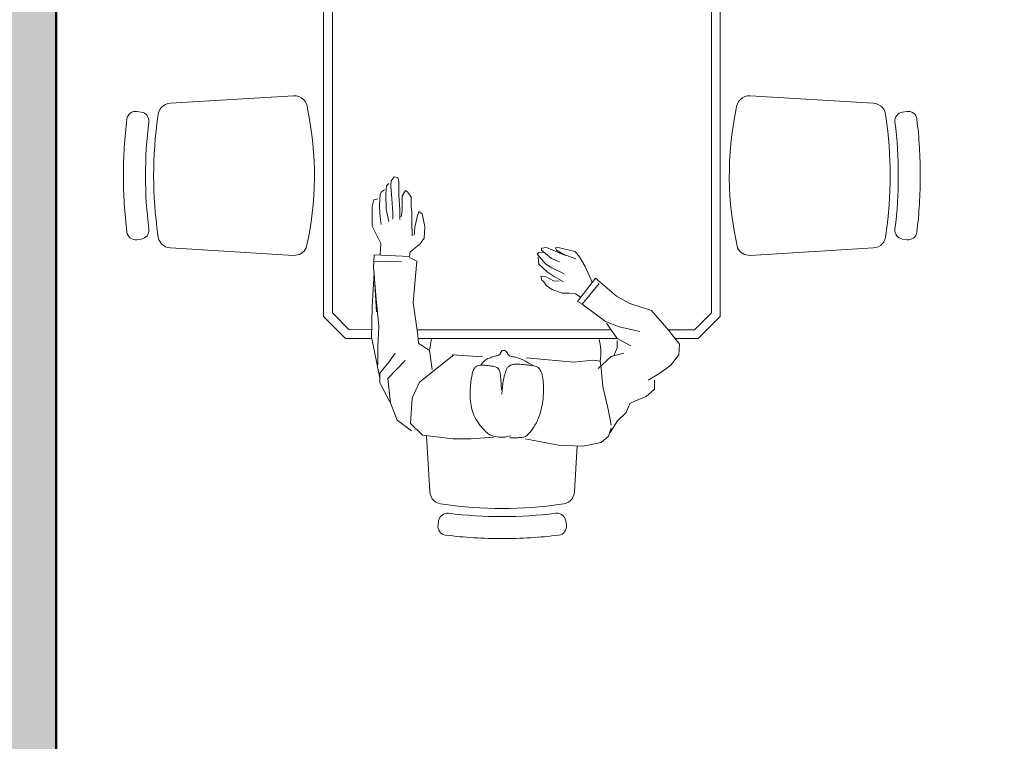
# Model space of a CAD drawing. Units: inches. Extents: x 1734 to 4011, y 1071 to 1891.
# Tile 6 of 27: x 1954 to 2022, y 1650 to 1699. Entities that reach past the tile are written whole.
import ezdxf

# ---------------------------------------------------------------- set-up
doc = ezdxf.new("R2010")
doc.units = ezdxf.units.IN
for name, color, linetype, lineweight in [('A-FURN', 8, 'Continuous', 18), ('A-WALL', 7, 'Continuous', 50), ('A-WALL-PATT', 8, 'Continuous', 13)]:
    doc.layers.add(name, color=color, linetype=linetype, lineweight=lineweight)

# ---------------------------------------------------------------- blocks, each defined once
blk = doc.blocks.new('A$C421907B3')
for p, q in [((0.7079, 2.565), (0.7245, 2.5796)), ((0.7245, 2.5796), (0.7652, 2.5876)), ((0.7652, 2.5876), (0.8209, 2.5856)), ((0.8209, 2.5856), (0.8965, 2.5714)), ((0.9684, 2.5672), (1.0195, 2.5715)), ((1.0195, 2.5715), (1.0607, 2.5715)), ((1.0607, 2.5715), (1.1301, 2.5633)), ((0.7038, 2.5568), (0.6875, 2.5302)), ((0.7017, 2.5468), (0.7079, 2.565)), ((0.8792, 2.5478), (0.8777, 2.5455)), ((0.8808, 2.55), (0.8792, 2.5478)), ((0.8823, 2.5521), (0.8808, 2.55)), ((0.8839, 2.5541), (0.8823, 2.5521)), ((0.8853, 2.556), (0.8839, 2.5541)), ((0.8868, 2.5577), (0.8853, 2.556)), ((0.8883, 2.5594), (0.8868, 2.5577)), ((0.8897, 2.5609), (0.8883, 2.5594)), ((0.8911, 2.5623), (0.8897, 2.5609)), ((0.8926, 2.5635), (0.8911, 2.5623)), ((0.8941, 2.5647), (0.8926, 2.5635)), ((0.8958, 2.5657), (0.8941, 2.5647)), ((0.8976, 2.5665), (0.8958, 2.5657)), ((0.8996, 2.5672), (0.8976, 2.5665)), ((0.9018, 2.5678), (0.8996, 2.5672)), ((0.9043, 2.5682), (0.9018, 2.5678)), ((0.9071, 2.5684), (0.9043, 2.5682)), ((0.9102, 2.5686), (0.9071, 2.5684)), ((0.9137, 2.5687), (0.9102, 2.5686)), ((0.9175, 2.5687), (0.9137, 2.5687)), ((0.9217, 2.5687), (0.9175, 2.5687)), ((0.9264, 2.5687), (0.9217, 2.5687)), ((0.9314, 2.5687), (0.9264, 2.5687)), ((0.9361, 2.5662), (0.9297, 2.5647)), ((0.942, 2.5671), (0.9361, 2.5662)), ((0.9475, 2.5676), (0.942, 2.5671)), ((0.9525, 2.5677), (0.9475, 2.5676)), ((0.9571, 2.5675), (0.9525, 2.5677)), ((0.9614, 2.5669), (0.9571, 2.5675)), ((0.9652, 2.5662), (0.9614, 2.5669)), ((0.9686, 2.5653), (0.9652, 2.5662)), ((0.9717, 2.5643), (0.9686, 2.5653)), ((0.9745, 2.5632), (0.9717, 2.5643)), ((0.977, 2.5619), (0.9745, 2.5632)), ((0.9794, 2.5605), (0.977, 2.5619)), ((0.9818, 2.5588), (0.9794, 2.5605)), ((0.9841, 2.5568), (0.9818, 2.5588)), ((0.9865, 2.5545), (0.9841, 2.5568)), ((0.9891, 2.5519), (0.9865, 2.5545)), ((0.9918, 2.5489), (0.9891, 2.5519)), ((0.9948, 2.5455), (0.9918, 2.5489)), ((1.1301, 2.5633), (1.1567, 2.5368)), ((1.1546, 2.5531), (1.1875, 2.5285)), ((0.6875, 2.5302), (0.6672, 2.5117)), ((0.7017, 2.5405), (0.7079, 2.5077)), ((0.8669, 2.5256), (0.8655, 2.522)), ((0.8684, 2.5289), (0.8669, 2.5256)), ((0.8699, 2.5321), (0.8684, 2.5289)), ((0.8714, 2.5351), (0.8699, 2.5321)), ((0.873, 2.5379), (0.8714, 2.5351)), ((0.8745, 2.5405), (0.873, 2.5379)), ((0.8761, 2.543), (0.8745, 2.5405)), ((0.8777, 2.5455), (0.8761, 2.543)), ((0.9978, 2.5419), (0.9948, 2.5455)), ((1.0008, 2.5379), (0.9978, 2.5419)), ((1.0037, 2.5338), (1.0008, 2.5379)), ((1.0066, 2.5294), (1.0037, 2.5338)), ((1.0093, 2.5249), (1.0066, 2.5294)), ((1.1567, 2.5368), (1.153, 2.4792)), ((1.1875, 2.5285), (1.202, 2.4895)), ((0.6672, 2.5117), (0.6589, 2.4912)), ((0.7079, 2.5077), (0.7204, 2.4524)), ((0.8604, 2.5049), (0.8594, 2.5001)), ((0.8616, 2.5096), (0.8604, 2.5049)), ((0.8628, 2.514), (0.8616, 2.5096)), ((0.8641, 2.5181), (0.8628, 2.514)), ((0.8655, 2.522), (0.8641, 2.5181)), ((1.0117, 2.5203), (1.0093, 2.5249)), ((1.0138, 2.5155), (1.0117, 2.5203)), ((1.0156, 2.5107), (1.0138, 2.5155)), ((1.0171, 2.5058), (1.0156, 2.5107)), ((1.0184, 2.5008), (1.0171, 2.5058)), ((0.6464, 2.4852), (0.6219, 2.4749)), ((0.6589, 2.4912), (0.6464, 2.4852)), ((0.8568, 2.4847), (0.8562, 2.4794)), ((0.8576, 2.49), (0.8568, 2.4847)), ((0.8584, 2.4951), (0.8576, 2.49)), ((0.8594, 2.5001), (0.8584, 2.4951)), ((1.0194, 2.4958), (1.0184, 2.5008)), ((1.0202, 2.4907), (1.0194, 2.4958)), ((1.0208, 2.4855), (1.0202, 2.4907)), ((1.0212, 2.4802), (1.0208, 2.4855)), ((1.202, 2.4895), (1.2083, 2.4342)), ((1.2041, 2.4875), (1.2266, 2.4445)), ((0.6219, 2.4749), (0.6036, 2.4584)), ((0.6036, 2.4584), (0.6036, 2.4379)), ((0.8552, 2.4632), (0.8551, 2.4579)), ((0.8554, 2.4686), (0.8552, 2.4632)), ((0.8558, 2.474), (0.8554, 2.4686)), ((0.8562, 2.4794), (0.8558, 2.474)), ((0.9483, 2.453), (0.9491, 2.4609)), ((0.9491, 2.4609), (0.9498, 2.4698)), ((0.9505, 2.4603), (0.9511, 2.447)), ((1.021, 2.4541), (1.0212, 2.4591)), ((1.0214, 2.4749), (1.0212, 2.4802)), ((1.0212, 2.4591), (1.0214, 2.4643)), ((1.0215, 2.4696), (1.0214, 2.4749)), ((1.0214, 2.4643), (1.0215, 2.4696)), ((1.153, 2.4792), (1.1364, 2.4424)), ((0.6178, 2.4379), (0.5933, 2.4236)), ((0.7204, 2.4524), (0.7246, 2.4114)), ((0.8551, 2.4579), (0.8552, 2.4527)), ((0.8552, 2.4527), (0.8554, 2.4476)), ((0.8554, 2.4476), (0.8557, 2.4428)), ((0.8557, 2.4428), (0.8561, 2.4383)), ((0.8561, 2.4383), (0.8567, 2.4341)), ((0.9455, 2.4346), (0.9465, 2.4399)), ((0.9465, 2.4399), (0.9474, 2.446)), ((0.9474, 2.446), (0.9483, 2.453)), ((0.9511, 2.447), (0.9518, 2.4364)), ((0.9518, 2.4364), (0.9526, 2.4283)), ((1.0186, 2.4325), (1.0192, 2.4362)), ((1.0192, 2.4362), (1.0197, 2.4402)), ((1.0197, 2.4402), (1.0202, 2.4445)), ((1.0202, 2.4445), (1.0206, 2.4492)), ((1.0206, 2.4492), (1.021, 2.4541)), ((1.1364, 2.4424), (1.0587, 2.3808)), ((1.2266, 2.4445), (1.2266, 2.422)), ((0.5933, 2.4236), (0.5667, 2.4051)), ((0.8567, 2.4341), (0.8574, 2.4301)), ((0.8574, 2.4301), (0.8582, 2.4265)), ((0.8582, 2.4265), (0.8591, 2.4232)), ((0.8591, 2.4232), (0.8601, 2.4202)), ((0.8601, 2.4202), (0.8612, 2.4176)), ((0.8612, 2.4176), (0.8624, 2.4152)), ((0.8624, 2.4152), (0.8637, 2.4132)), ((0.9391, 2.4131), (0.9399, 2.415)), ((0.9399, 2.415), (0.9408, 2.4171)), ((0.9408, 2.4171), (0.9416, 2.4196)), ((0.9416, 2.4196), (0.9425, 2.4226)), ((0.9425, 2.4226), (0.9435, 2.426)), ((0.9435, 2.426), (0.9445, 2.43)), ((0.9445, 2.43), (0.9455, 2.4346)), ((0.9526, 2.4283), (0.9535, 2.4222)), ((0.9535, 2.4222), (0.9546, 2.4177)), ((0.9546, 2.4177), (0.9558, 2.4146)), ((0.9558, 2.4146), (0.9572, 2.4124)), ((1.0124, 2.4119), (1.0135, 2.4137)), ((1.0135, 2.4137), (1.0144, 2.4158)), ((1.0144, 2.4158), (1.0152, 2.418)), ((1.0152, 2.418), (1.016, 2.4204)), ((1.016, 2.4204), (1.0168, 2.423)), ((1.0168, 2.423), (1.0174, 2.4259)), ((1.0174, 2.4259), (1.0181, 2.429)), ((1.0181, 2.429), (1.0186, 2.4325)), ((1.1077, 2.4136), (1.114, 2.3706)), ((1.2083, 2.4342), (1.1693, 2.3932)), ((1.2266, 2.422), (1.2062, 2.3974)), ((1.2447, 2.3435), (1.2266, 2.4332)), ((0.5667, 2.4051), (0.5484, 2.3805)), ((0.7308, 2.4114), (0.7018, 2.3846)), ((0.7246, 2.4114), (0.7267, 2.3949)), ((0.7267, 2.3949), (0.7429, 2.3929)), ((0.7429, 2.3929), (0.7861, 2.3972)), ((0.7861, 2.3972), (0.8946, 2.387)), ((0.8637, 2.4132), (0.8651, 2.4114)), ((0.8651, 2.4114), (0.8666, 2.41)), ((0.8666, 2.41), (0.8682, 2.4088)), ((0.8682, 2.4088), (0.87, 2.4078)), ((0.87, 2.4078), (0.872, 2.407)), ((0.872, 2.407), (0.8742, 2.4063)), ((0.8742, 2.4063), (0.8767, 2.4058)), ((0.8767, 2.4058), (0.8794, 2.4052)), ((0.8794, 2.4052), (0.8824, 2.4048)), ((0.8801, 2.4042), (0.8884, 2.3992)), ((0.8824, 2.4048), (0.8857, 2.4043)), ((0.8857, 2.4043), (0.8891, 2.4039)), ((0.8884, 2.3992), (0.8957, 2.3952)), ((0.8891, 2.4039), (0.8925, 2.4035)), ((0.8925, 2.4035), (0.896, 2.4031)), ((0.8957, 2.3952), (0.9019, 2.3921)), ((0.896, 2.4031), (0.8995, 2.4027)), ((0.8995, 2.4027), (0.9028, 2.4024)), ((0.9019, 2.3921), (0.9073, 2.3897)), ((0.9028, 2.4024), (0.9059, 2.4022)), ((0.9059, 2.4022), (0.9088, 2.4019)), ((0.9088, 2.4019), (0.9114, 2.4018)), ((0.9114, 2.4018), (0.9138, 2.4016)), ((0.9138, 2.4016), (0.9161, 2.4016)), ((0.9161, 2.4016), (0.9182, 2.4016)), ((0.9182, 2.4016), (0.9201, 2.4017)), ((0.9201, 2.4017), (0.9219, 2.4019)), ((0.9219, 2.4019), (0.9237, 2.4022)), ((0.9237, 2.4022), (0.9254, 2.4026)), ((0.9254, 2.4026), (0.927, 2.4031)), ((0.927, 2.4031), (0.9286, 2.4037)), ((0.9286, 2.4037), (0.9301, 2.4044)), ((0.9301, 2.4044), (0.9315, 2.4052)), ((0.9315, 2.4052), (0.9329, 2.406)), ((0.9329, 2.406), (0.9341, 2.4069)), ((0.9341, 2.4069), (0.9353, 2.4079)), ((0.9353, 2.4079), (0.9363, 2.409)), ((0.9363, 2.409), (0.9373, 2.4102)), ((0.9373, 2.4102), (0.9382, 2.4116)), ((0.9382, 2.4116), (0.9391, 2.4131)), ((0.9572, 2.4124), (0.9588, 2.4109)), ((0.9588, 2.4109), (0.9606, 2.4096)), ((0.9606, 2.4096), (0.9626, 2.4086)), ((0.9626, 2.4086), (0.9647, 2.4077)), ((0.9647, 2.4077), (0.9671, 2.407)), ((0.9671, 2.407), (0.9696, 2.4064)), ((0.9696, 2.4064), (0.9722, 2.406)), ((0.9722, 2.406), (0.9751, 2.4055)), ((0.9751, 2.4055), (0.9781, 2.4052)), ((0.9781, 2.4052), (0.9812, 2.4048)), ((0.9812, 2.4048), (0.9844, 2.4045)), ((0.9837, 2.3905), (0.9863, 2.3922)), ((0.9844, 2.4045), (0.9877, 2.4043)), ((0.9863, 2.3922), (0.9889, 2.3941)), ((0.9877, 2.4043), (0.9909, 2.4041)), ((0.9889, 2.3941), (0.9915, 2.3965)), ((0.9909, 2.4041), (0.9941, 2.4041)), ((0.9915, 2.3965), (0.994, 2.3993)), ((0.994, 2.3993), (0.9965, 2.4026)), ((0.9941, 2.4041), (0.9971, 2.4042)), ((0.9971, 2.4042), (0.9999, 2.4044)), ((0.9999, 2.4044), (1.0025, 2.4049)), ((1.0025, 2.4049), (1.0047, 2.4055)), ((1.0047, 2.4055), (1.0067, 2.4064)), ((1.0067, 2.4064), (1.0085, 2.4075)), ((1.0085, 2.4075), (1.01, 2.4087)), ((1.01, 2.4087), (1.0113, 2.4102)), ((1.0113, 2.4102), (1.0124, 2.4119)), ((1.2062, 2.3974), (1.1917, 2.3769)), ((1.2308, 2.3624), (1.2308, 2.4035)), ((0.5484, 2.3805), (0.5463, 2.356)), ((0.7018, 2.3846), (0.6731, 2.3766)), ((0.6876, 2.3643), (0.6959, 2.3826)), ((0.9073, 2.3897), (0.9119, 2.3881)), ((0.9119, 2.3881), (0.9157, 2.3869)), ((0.9157, 2.3869), (0.919, 2.386)), ((0.919, 2.386), (0.9217, 2.3854)), ((0.9217, 2.3854), (0.924, 2.3849)), ((0.924, 2.3849), (0.926, 2.3844)), ((0.926, 2.3844), (0.9277, 2.384)), ((0.9277, 2.384), (0.929, 2.3837)), ((0.929, 2.3837), (0.9302, 2.3833)), ((0.9302, 2.3833), (0.9312, 2.383)), ((0.9312, 2.383), (0.932, 2.3826)), ((0.932, 2.3826), (0.9327, 2.3823)), ((0.9327, 2.3823), (0.9334, 2.3818)), ((0.9334, 2.3818), (0.934, 2.3813)), ((0.934, 2.3813), (0.9346, 2.3808)), ((0.9346, 2.3808), (0.9351, 2.3803)), ((0.9351, 2.3803), (0.9356, 2.3797)), ((0.9356, 2.3797), (0.936, 2.379)), ((0.936, 2.379), (0.9365, 2.3783)), ((0.9365, 2.3783), (0.9369, 2.3776)), ((0.9369, 2.3776), (0.9372, 2.3769)), ((0.9372, 2.3769), (0.9376, 2.3761)), ((0.9376, 2.3761), (0.938, 2.3753)), ((0.938, 2.3753), (0.9384, 2.3746)), ((0.9384, 2.3746), (0.9389, 2.3738)), ((0.9389, 2.3738), (0.9395, 2.3731)), ((0.9395, 2.3731), (0.9401, 2.3725)), ((0.9401, 2.3725), (0.9408, 2.3719)), ((0.9408, 2.3719), (0.9417, 2.3714)), ((0.9417, 2.3714), (0.9426, 2.371)), ((0.9426, 2.371), (0.9437, 2.3707)), ((0.9437, 2.3707), (0.9447, 2.3706)), ((0.9447, 2.3706), (0.9458, 2.3705)), ((0.9458, 2.3705), (0.9468, 2.3706)), ((0.9468, 2.3706), (0.9478, 2.3708)), ((0.9478, 2.3708), (0.9487, 2.3712)), ((0.9487, 2.3712), (0.9494, 2.3717)), ((0.9494, 2.3717), (0.9501, 2.3723)), ((0.9501, 2.3723), (0.9507, 2.3731)), ((0.9507, 2.3731), (0.9512, 2.3739)), ((0.9512, 2.3739), (0.9517, 2.3747)), ((0.9517, 2.3747), (0.9521, 2.3755)), ((0.9521, 2.3755), (0.9524, 2.3764)), ((0.9524, 2.3764), (0.9527, 2.3771)), ((0.9527, 2.3771), (0.953, 2.3778)), ((0.953, 2.3778), (0.9533, 2.3785)), ((0.9533, 2.3785), (0.9536, 2.379)), ((0.9536, 2.379), (0.954, 2.3796)), ((0.954, 2.3796), (0.9546, 2.3801)), ((0.9546, 2.3801), (0.9554, 2.3805)), ((0.9554, 2.3805), (0.9564, 2.381)), ((0.9564, 2.381), (0.9577, 2.3815)), ((0.9577, 2.3815), (0.9593, 2.382)), ((0.9593, 2.382), (0.9611, 2.3826)), ((0.9611, 2.3826), (0.9632, 2.3832)), ((0.9632, 2.3832), (0.9655, 2.3838)), ((0.9655, 2.3838), (0.9679, 2.3845)), ((0.9679, 2.3845), (0.9705, 2.3853)), ((0.9705, 2.3853), (0.9731, 2.3861)), ((0.9731, 2.3861), (0.9757, 2.387)), ((0.9757, 2.387), (0.9784, 2.388)), ((0.9784, 2.388), (0.9811, 2.3892)), ((0.9811, 2.3892), (0.9837, 2.3905)), ((0.9931, 2.3848), (1.0625, 2.3808)), ((1.114, 2.3706), (1.1095, 2.3436)), ((1.114, 2.3706), (1.1385, 2.3544)), ((0.5463, 2.356), (0.5709, 2.3252)), ((0.6569, 2.3601), (0.6876, 2.3438)), ((0.6876, 2.3478), (0.6876, 2.3643)), ((1.1385, 2.3544), (1.1406, 2.3358)), ((1.2287, 2.3154), (1.2308, 2.3624)), ((0.5709, 2.3252), (0.6099, 2.2802)), ((0.6835, 2.317), (0.6365, 2.3273)), ((0.6876, 2.3438), (0.7122, 2.3088)), ((1.1406, 2.3358), (1.151, 2.262)), ((0.7143, 2.3048), (0.6835, 2.317)), ((0.7674, 2.2656), (0.7143, 2.3048)), ((1.235, 2.2538), (1.2287, 2.3154)), ((0.6099, 2.2802), (0.659, 2.2637)), ((0.659, 2.2637), (0.6898, 2.2475)), ((0.7288, 2.2187), (0.7675, 2.2658)), ((0.7779, 2.2598), (0.7368, 2.2065)), ((0.7675, 2.2658), (0.7779, 2.2598)), ((1.151, 2.262), (1.1428, 2.1677)), ((0.6898, 2.2475), (0.7368, 2.2065)), ((0.7716, 2.2487), (0.7827, 2.2421)), ((0.7827, 2.2421), (0.7969, 2.2406)), ((0.7969, 2.2406), (0.8131, 2.2406)), ((0.8131, 2.2406), (0.8354, 2.2325)), ((1.2413, 2.1822), (1.235, 2.2538)), ((0.7509, 2.2021), (0.7458, 2.2146)), ((0.8094, 2.2146), (0.8309, 2.2028)), ((0.8324, 2.2124), (0.8198, 2.2132)), ((0.8494, 2.2036), (0.8324, 2.2124)), ((0.8354, 2.2325), (0.8487, 2.2236)), ((0.8487, 2.2236), (0.8546, 2.2147)), ((0.8546, 2.2147), (0.859, 2.211)), ((0.7606, 2.1798), (0.7509, 2.2021)), ((0.8079, 2.1969), (0.8361, 2.1828)), ((0.8309, 2.2028), (0.8472, 2.1925)), ((0.8472, 2.1925), (0.8658, 2.1747)), ((0.8613, 2.2021), (0.8494, 2.2036)), ((0.859, 2.211), (0.8613, 2.2021)), ((0.7732, 2.1583), (0.7606, 2.1798)), ((0.8191, 2.1695), (0.8369, 2.1621)), ((0.8361, 2.1828), (0.8502, 2.1747)), ((0.8502, 2.1747), (0.8695, 2.1518)), ((0.8658, 2.1747), (0.8672, 2.1591)), ((1.1428, 2.1677), (1.159, 2.1597)), ((1.1777, 2.1697), (1.2413, 2.1677)), ((1.2392, 2.1535), (1.2413, 2.1822)), ((0.7835, 2.1457), (0.7732, 2.1583)), ((0.7814, 2.1628), (0.8102, 2.1517)), ((0.8221, 2.1369), (0.7835, 2.1457)), ((0.848, 2.1369), (0.805, 2.1547)), ((0.8102, 2.1517), (0.8257, 2.1428)), ((0.8369, 2.1621), (0.8599, 2.1429)), ((0.8658, 2.1481), (0.8561, 2.1473)), ((0.8695, 2.1518), (0.8658, 2.1481)), ((1.158, 2.1467), (1.1354, 2.1286)), ((1.1595, 2.1573), (1.158, 2.1467)), ((1.1595, 2.1573), (1.2392, 2.1535)), ((1.226, 2.1528), (1.2245, 2.1279)), ((0.828, 2.1376), (0.8221, 2.1369)), ((0.8257, 2.1428), (0.828, 2.1376)), ((0.8599, 2.1384), (0.848, 2.1369)), ((0.8599, 2.1429), (0.8599, 2.1384)), ((1.1354, 2.1286), (1.1263, 2.1158)), ((1.2245, 2.1279), (1.2358, 2.1052)), ((1.1263, 2.1158), (1.1248, 2.0893)), ((1.1474, 2.0909), (1.149, 2.1089)), ((1.1535, 2.1105), (1.1536, 2.078)), ((1.2358, 2.1052), (1.2442, 2.0886)), ((1.1248, 2.0893), (1.1308, 2.0606)), ((1.1414, 2.0644), (1.1474, 2.0909)), ((1.2238, 2.0848), (1.2269, 2.0606)), ((1.2442, 2.0886), (1.2442, 2.0441)), ((1.1308, 2.0606), (1.1377, 2.0553)), ((1.1377, 2.0553), (1.1414, 2.0644)), ((1.1536, 2.078), (1.1543, 2.0568)), ((1.1543, 2.0568), (1.1551, 2.0432)), ((1.1762, 2.0539), (1.1784, 2.0674)), ((1.1815, 2.0735), (1.1815, 2.0516)), ((1.1974, 2.0584), (1.1974, 2.0727)), ((1.1996, 2.0267), (1.1974, 2.0584)), ((1.2064, 2.078), (1.2125, 2.0501)), ((1.2269, 2.0606), (1.2276, 2.0418)), ((1.1551, 2.0432), (1.1558, 2.0229)), ((1.1762, 2.0357), (1.1762, 2.0539)), ((1.1762, 2.0206), (1.1762, 2.0357)), ((1.1815, 2.0516), (1.1831, 2.0183)), ((1.2125, 2.0501), (1.2132, 2.0154)), ((1.2276, 2.0418), (1.2261, 2.0161)), ((1.2442, 2.0441), (1.2404, 2.029)), ((1.1558, 2.0229), (1.1641, 2.0108)), ((1.168, 2.0077), (1.1762, 2.0206)), ((1.1831, 2.0183), (1.1831, 1.9874)), ((1.2019, 1.9979), (1.1996, 2.0267)), ((1.2132, 2.0154), (1.2117, 1.9972)), ((1.2261, 2.0161), (1.223, 2.0108)), ((1.2404, 2.029), (1.2314, 2.0267)), ((1.1641, 2.0108), (1.168, 2.0077)), ((1.2012, 1.9859), (1.2019, 1.9979)), ((1.2117, 1.9972), (1.2064, 1.9919)), ((1.223, 2.0108), (1.2163, 2.0063)), ((1.1831, 1.9874), (1.186, 1.9783)), ((1.186, 1.9783), (1.1944, 1.9768)), ((1.1944, 1.9768), (1.2012, 1.9859))]:
    blk.add_line(p, q)
at = {"ltscale": 0.1}
for points in [[(0.9489, 2.7478, 0.030867), (0.827, 2.7403, -0.408428), (0.8047, 2.7573), (0.8033, 2.7672, -0.419966), (0.8206, 2.7899, -0.030916), (0.9489, 2.7978, -0.030916), (1.0772, 2.7899, -0.419966), (1.0945, 2.7672), (1.0931, 2.7573, -0.408428), (1.0708, 2.7403, 0.030867)], [(0.0782, 2.1079, -0.399285), (0.1067, 2.1378), (0.3861, 2.1548, -0.305593), (0.4148, 2.1375, -0.109362), (0.4176, 1.8225, -0.429301), (0.3861, 1.7925), (0.1067, 1.8094, -0.399285), (0.0782, 1.8394, -0.071734)], [(1.7302, 2.1079, 0.399285), (1.7017, 2.1378), (1.4223, 2.1548, 0.305593), (1.3936, 2.1375, 0.109362), (1.3908, 1.8225, 0.429301), (1.4223, 1.7925), (1.7017, 1.8094, 0.399285), (1.7302, 1.8394, 0.071734)], [(0.05, 1.9736, 0.030867), (0.0575, 1.8517, -0.408428), (0.0405, 1.8294), (0.0306, 1.828, -0.419966), (0.0079, 1.8453, -0.030916), (0, 1.9736, -0.030916), (0.0079, 2.1019, -0.419966), (0.0306, 2.1193), (0.0405, 2.1178, -0.408428), (0.0575, 2.0956, 0.030867)], [(1.7584, 1.9736, -0.030867), (1.7509, 1.8517, 0.408428), (1.7679, 1.8294), (1.7778, 1.828, 0.419966), (1.8005, 1.8453, 0.030916), (1.8084, 1.9736, 0.030916), (1.8005, 2.1019, 0.419966), (1.7778, 2.1193), (1.7679, 2.1178, 0.408428), (1.7509, 2.0956, -0.030867)]]:
    blk.add_lwpolyline(points, format="xyb", close=True, dxfattribs=at)
blk.add_lwpolyline([(0.7784, 2.5871), (0.7847, 2.6911, -0.399285), (0.8147, 2.7196, -0.071734), (1.0831, 2.7196, -0.399285), (1.1131, 2.6911), (1.1208, 2.5644)], format="xyb", dxfattribs=at)
for points in [[(0.4542, 1.2262), (0.4542, 2.2936), (0.5042, 2.3436), (0.5562, 2.3436)], [(0.6878, 2.3436), (1.1397, 2.3436)], [(1.2446, 2.3436), (1.3042, 2.3436), (1.3542, 2.2936), (1.3542, 1.0533)], [(0.4742, 1.2101), (0.4742, 2.2853), (0.5125, 2.3236), (0.5723, 2.3236)], [(0.7018, 2.3236), (1.1423, 2.3236)], [(1.245, 2.3234), (1.2959, 2.3236), (1.3342, 2.2853), (1.3342, 1.0419)]]:
    blk.add_lwpolyline(points, dxfattribs=at)
blk.add_lwpolyline([(1.2332, 2.2712), (1.2341, 2.2831), (1.2396, 2.1946), (1.2396, 2.1946), (1.2419, 2.2332), (1.2437, 2.2711), (1.2448, 2.3081), (1.2452, 2.3436)])
blk.add_arc((0.8297, 2.3756), 0.1048, 169.4107, 197.7809)

msp = doc.modelspace()

# ---------------------------------------------------------------- hatches: boundary and pattern name
at = {"layer": 'A-WALL-PATT'}
h = msp.add_hatch(color=256, dxfattribs=at)
h.dxf.hatch_style = 1
h.paths.add_polyline_path([(1857.65, 1835.061), (1857.65, 1793.061), (1862.65, 1793.061), (1862.65, 1835.061), (1951.65, 1835.061), (1951.65, 1763.061), (1897.65, 1763.061), (1897.65, 1758.061), (1951.65, 1758.061), (1951.65, 1617.061), (1956.65, 1617.061), (1956.65, 1758.061), (2009.65, 1758.061), (2009.65, 1763.061), (1956.65, 1763.061), (1956.65, 1835.061), (2044.65, 1835.061), (2044.65, 1763.061), (2039.65, 1763.061), (2039.65, 1758.061), (2054.65, 1758.061), (2054.65, 1763.061), (2049.65, 1763.061), (2049.65, 1835.061), (2109.65, 1835.061), (2109.65, 1763.061), (2084.65, 1763.061), (2084.65, 1758.061), (2109.65, 1758.061), (2109.65, 1530.061), (2095.15, 1530.061), (2095.15, 1525.061), (2109.65, 1525.061), (2109.65, 1471.061), (2089.15, 1471.061), (2089.15, 1466.061), (2109.65, 1466.061), (2109.65, 1250.061), (2015.65, 1250.061), (2015.65, 1241.061), (2109.65, 1241.061), (2109.65, 1133.061), (1952.65, 1133.061), (1952.65, 1197.061), (1953.65, 1197.061), (1953.65, 1202.061), (1946.65, 1202.061), (1946.65, 1133.061), (1934.65, 1133.061), (1934.65, 1124.061), (2118.65, 1124.061), (2118.65, 1844.061), (1758.65, 1844.061), (1758.65, 1758.061), (1773.65, 1758.061), (1773.65, 1763.061), (1767.65, 1763.061), (1767.65, 1835.061)])
h.paths.add_polyline_path([(1803.65, 1649.061), (1812.65, 1649.061), (1812.65, 1758.061), (1867.65, 1758.061), (1867.65, 1763.061), (1797.65, 1763.061), (1797.65, 1758.061), (1803.65, 1758.061)], flags=17)
h.paths.add_polyline_path([(1803.65, 1572.061), (1956.65, 1572.061), (1956.65, 1581.061), (1951.65, 1581.061), (1951.65, 1577.061), (1812.65, 1577.061), (1812.65, 1601.061), (1803.65, 1601.061)], flags=17)
h.paths.add_polyline_path([(2044.65, 1530.061), (2044.65, 1525.061), (2059.15, 1525.061), (2059.15, 1530.061)], flags=17)
h.paths.add_polyline_path([(2009.65, 1466.061), (2035.15, 1466.061), (2035.15, 1471.061), (2014.65, 1471.061), (2014.65, 1530.061), (2009.65, 1530.061)], flags=17)
h.paths.add_polyline_path([(1896.65, 1537.061), (1896.65, 1533.061), (1901.65, 1533.061), (1901.65, 1542.061), (1803.65, 1542.061), (1803.65, 1507.061), (1812.65, 1507.061), (1812.65, 1537.061)], flags=17)
h.paths.add_polyline_path([(1906.65, 1466.061), (1906.65, 1471.061), (1901.65, 1471.061), (1901.65, 1503.061), (1896.65, 1503.061), (1896.65, 1471.061), (1812.65, 1471.061), (1812.65, 1483.061), (1803.65, 1483.061), (1803.65, 1400.061), (1812.65, 1400.061), (1812.65, 1466.061)], flags=17)
h.paths.add_polyline_path([(1951.65, 1334.061), (1909.15, 1334.061), (1909.15, 1325.061), (1956.65, 1325.061), (1956.65, 1466.061), (1961.65, 1466.061), (1961.65, 1471.061), (1942.65, 1471.061), (1942.65, 1466.061), (1951.65, 1466.061)], flags=17)
h.paths.add_polyline_path([(1812.65, 1334.061), (1812.65, 1352.061), (1803.65, 1352.061), (1803.65, 1325.061), (1855.15, 1325.061), (1855.15, 1334.061)], flags=17)
h.paths.add_polyline_path([(1956.65, 1298.061), (1956.65, 1301.061), (1947.65, 1301.061), (1947.65, 1298.061)], flags=17)
h.paths.add_polyline_path([(1967.65, 1241.061), (1967.65, 1250.061), (1947.65, 1250.061), (1947.65, 1241.061)], flags=17)

# ---------------------------------------------------------------- linework, layer by layer
at = {"layer": 'A-WALL'}
msp.add_line((1956.65, 1617.061), (1956.65, 1758.061), dxfattribs=at)

# ---------------------------------------------------------------- block references
at = {"layer": 'A-FURN', "xscale": 30.26057373645948, "yscale": 30.26057373645948, "zscale": 30.26057373645948, "rotation": 180}
msp.add_blockref('A$C421907B3', (2015.998, 1748.475), dxfattribs=at)

doc.saveas('drawing.dxf')
